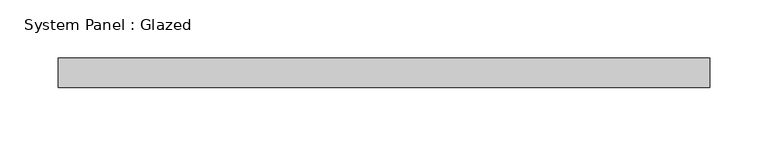
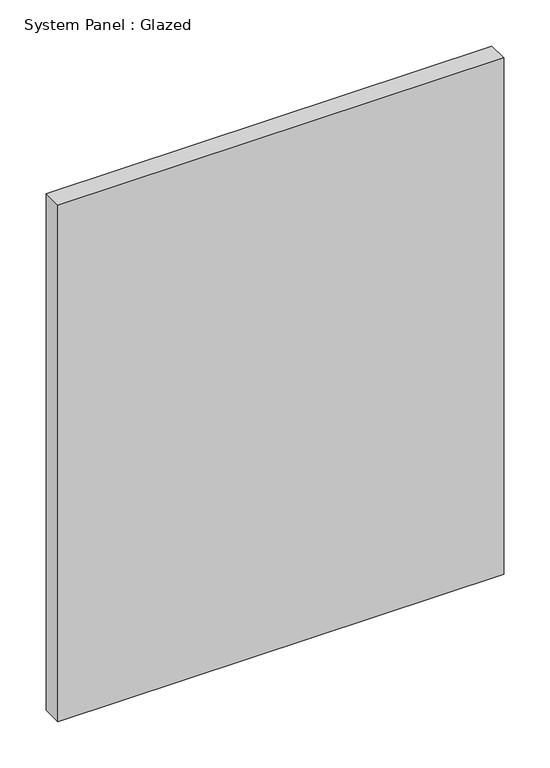
"""IFC4 building model written with IfcOpenShell, lengths in millimetres: plate geometry, System Panel : Glazed."""

from ifc_helpers import new_model, si_unit, origin, origin_with_axes, place, context, project, spatial, polyline, outline, extrude, source, transform, mapped, element, save


def system_panel_glazed_ea517728(model_context):
    return source(origin(), model_context, "Body", "SweptSolid", [
        extrude(outline(polyline([(279.4, 19.05), (-279.4, 19.05), (-279.4, 44.45), (279.4, 44.45), (279.4, 19.05)])), origin_with_axes(), (0.0, 0.0, 1.0), 684.6823007),
    ])


if __name__ == "__main__":
    model = new_model("IFC4")
    model_context = context("Model", 3, world=origin())
    ifc_project = project(units=[si_unit("LENGTHUNIT", "METRE", prefix="MILLI")], contexts=[model_context])
    site = spatial("IfcSite", under=ifc_project)
    building = spatial("IfcBuilding", under=site)
    placement = place(None, origin())
    system_panel_glazed_shape = system_panel_glazed_ea517728(model_context)
    element("IfcPlate", 1, ObjectType="System Panel : Glazed", at=placement, inside=building, context=model_context, shape_type="MappedRepresentation", body=[
        mapped(system_panel_glazed_shape, transform((0.0, 0.0, 0.0), x_axis=(1.0, 0.0, 0.0), y_axis=(0.0, 1.0, 0.0), z_axis=(0.0, 0.0, 1.0))),
    ])
    save(model, "model.ifc")

# Revit data of these elements
# Type "System Panel : Glazed"
#   Construction Type Id = "GSP4R"
#   Analytic Construction = "1/8 in Pilkington single glazing"
#   Visual Light Transmittance = 0.9
#   Solar Heat Gain Coefficient = 0.86
#   Heat Transfer Coefficient (U) = 1.18115 BTU/(h·ft²·°F)
#   Define Thermal Properties by = 1
# Element 1 (IfcPlate, "System Panel : Glazed")
#   Materials on its faces: "Glass"
# Materials
#   "Glass": class "Glass", colour RGB 0 128 192, transparency 0.75, Description = "Soda Lime Glass", Cost = 0
